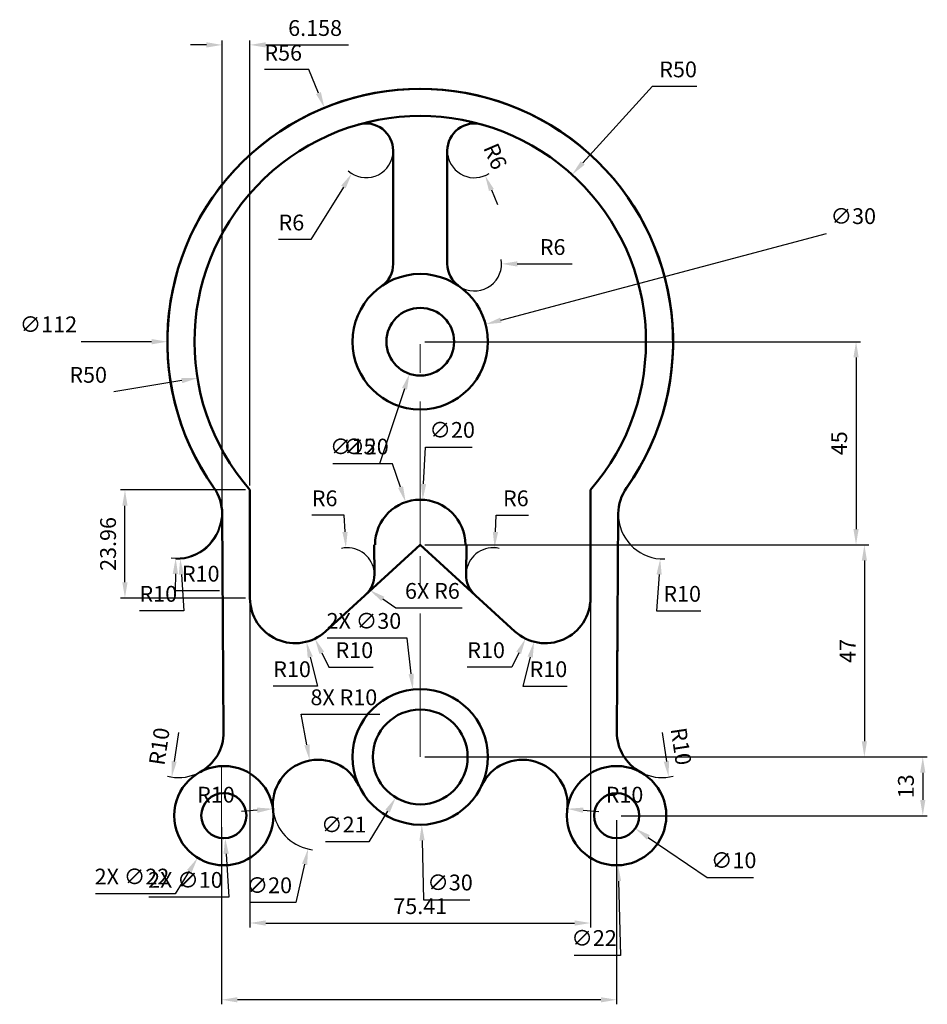
# Model space of a CAD drawing. Units: millimetres. Extents: x 3612 to 3813, y 660 to 878.
import ezdxf

# ---------------------------------------------------------------- set-up
doc = ezdxf.new("R2010")
doc.units = ezdxf.units.MM
doc.linetypes.add('CENTER', pattern=[50.8, 31.75, -6.35, 6.35, -6.35])
for name, color, linetype, lineweight in [('M-CNTR', 4, 'CENTER', 18), ('M-CONS', 8, 'Continuous', 13), ('M-DIMS', 3, 'Continuous', 25), ('M-OUTL', 7, 'Continuous', 50)]:
    doc.layers.add(name, color=color, linetype=linetype, lineweight=lineweight)
doc.styles.get("Standard").update_dxf_attribs({"font": 'arial.ttf'})
doc.dimstyles.new('AM_ISO$0', dxfattribs={"dimtxt": 3.5, "dimasz": 3.5, "dimexe": 1, "dimexo": 1, "dimgap": 1.5, "dimtad": 1, "dimdsep": 46, "dimtxsty": 'Standard', "dimcen": 0, "dimclrd": 256, "dimclre": 256, "dimclrt": 2, "dimadec": 0, "dimazin": 2, "dimtp": 0.1, "dimtm": 0.1, "dimtfac": 0.71, "dimtdec": 3, "dimtmove": 0, "dimatfit": 3, "dimfxl": 1, "dimlwd": -1, "dimlwe": -1, "dimarcsym": 1})
doc.dimstyles.new('AM_ISO$3', dxfattribs={"dimtxt": 3.5, "dimasz": 3.5, "dimexe": 1, "dimexo": 1, "dimgap": 1.5, "dimtad": 1, "dimtoh": 1, "dimdsep": 46, "dimtxsty": 'Standard', "dimcen": 0, "dimclrd": 256, "dimclre": 256, "dimclrt": 2, "dimadec": 0, "dimazin": 2, "dimtp": 0.1, "dimtm": 0.1, "dimtfac": 0.71, "dimtdec": 3, "dimtofl": 0, "dimtmove": 0, "dimatfit": 0, "dimfxl": 1, "dimlwd": -1, "dimlwe": -1, "dimarcsym": 1})
doc.dimstyles.new('AM_ISO$4', dxfattribs={"dimtxt": 3.5, "dimasz": 3.5, "dimexe": 1, "dimexo": 1, "dimgap": 1.5, "dimtad": 1, "dimtoh": 1, "dimdsep": 46, "dimtxsty": 'Standard', "dimcen": 0, "dimclrd": 256, "dimclre": 256, "dimclrt": 2, "dimadec": 0, "dimazin": 2, "dimtp": 0.1, "dimtm": 0.1, "dimtfac": 0.71, "dimtdec": 3, "dimtofl": 0, "dimtmove": 0, "dimatfit": 0, "dimfxl": 1, "dimlwd": -1, "dimlwe": -1, "dimarcsym": 1})

# ---------------------------------------------------------------- blocks, each defined once
blk = doc.blocks.new('*D3')
at = {"layer": 'Defpoints', "color": 0, "transparency": 16777216}
for p in [(3723.75, 703.9), (3733.71, 703.03)]:
    blk.add_point(p, dxfattribs=at)
at = {"layer": 'M-DIMS', "color": 0, "linetype": 'ByBlock', "transparency": 16777216}
blk.add_line((3737.2, 702.72), (3740.69, 702.41), dxfattribs=at)
at = {"layer": 'M-DIMS', "color": 0, "transparency": 16777216}
blk.add_solid([(3737.25, 703.3), (3737.15, 702.14), (3733.71, 703.03)], dxfattribs=at)
at = {"layer": 'M-DIMS', "color": 0, "transparency": 16777216, "insert": (3746.36, 705.7), "char_height": 3.5, "attachment_point": 5}
blk.add_mtext('R10', dxfattribs=at)
blk = doc.blocks.new('*D4')
at = {"layer": 'Defpoints', "color": 0, "transparency": 16777216}
for p in [(3689.12, 848.84), (3685.95, 843.75)]:
    blk.add_point(p, dxfattribs=at)
at = {"layer": 'M-DIMS', "color": 0, "linetype": 'ByBlock', "transparency": 16777216}
for p, q in [((3684.11, 840.77), (3676.9, 829.17)), ((3676.9, 829.17), (3669.76, 829.17))]:
    blk.add_line(p, q, dxfattribs=at)
blk.add_arc((3689.12, 848.84), 6, 228.6118, 350.4507, dxfattribs=at)
at = {"layer": 'M-DIMS', "color": 0, "transparency": 16777216}
blk.add_solid([(3683.61, 841.08), (3684.6, 840.47), (3685.95, 843.75)], dxfattribs=at)
at = {"layer": 'M-DIMS', "color": 0, "transparency": 16777216, "insert": (3672.58, 832.46), "char_height": 3.5, "attachment_point": 5}
blk.add_mtext('R6', dxfattribs=at)
blk = doc.blocks.new('*D5')
at = {"layer": 'Defpoints', "color": 0, "transparency": 16777216}
for p in [(3754.67, 719.95), (3756.15, 710.06)]:
    blk.add_point(p, dxfattribs=at)
at = {"layer": 'M-DIMS', "color": 0, "linetype": 'ByBlock', "transparency": 16777216}
blk.add_line((3754.67, 719.95), (3755.63, 713.52), dxfattribs=at)
blk.add_arc((3754.67, 719.95), 10, 247.141, 284.2413, dxfattribs=at)
at = {"layer": 'M-DIMS', "color": 0, "transparency": 16777216}
blk.add_solid([(3756.2, 713.61), (3755.05, 713.44), (3756.15, 710.06)], dxfattribs=at)
at = {"layer": 'M-DIMS', "color": 0, "transparency": 16777216, "insert": (3758.46, 716.8), "char_height": 3.5, "attachment_point": 5, "rotation": 278.5117}
blk.add_mtext('R10', dxfattribs=at)
blk = doc.blocks.new('*D6')
at = {"layer": 'Defpoints', "color": 0, "transparency": 16777216}
for p in [(3754.98, 768.37), (3754.27, 758.4)]:
    blk.add_point(p, dxfattribs=at)
at = {"layer": 'M-DIMS', "color": 0, "linetype": 'ByBlock', "transparency": 16777216}
for p, q in [((3754.02, 754.91), (3753.45, 746.91)), ((3753.45, 746.91), (3763.3, 746.91))]:
    blk.add_line(p, q, dxfattribs=at)
blk.add_arc((3754.98, 768.37), 10, 185.3551, 271.654, dxfattribs=at)
at = {"layer": 'M-DIMS', "color": 0, "transparency": 16777216}
blk.add_solid([(3753.44, 754.95), (3754.6, 754.87), (3754.27, 758.4)], dxfattribs=at)
at = {"layer": 'M-DIMS', "color": 0, "transparency": 16777216, "insert": (3759.13, 750.2), "char_height": 3.5, "attachment_point": 5}
blk.add_mtext('R10', dxfattribs=at)
blk = doc.blocks.new('*D7')
at = {"layer": 'Defpoints', "color": 0, "transparency": 16777216}
for p in [(3647.12, 768.57), (3646.95, 758.57)]:
    blk.add_point(p, dxfattribs=at)
at = {"layer": 'M-DIMS', "color": 0, "linetype": 'ByBlock', "transparency": 16777216}
for p, q in [((3646.89, 755.07), (3646.82, 751.37)), ((3646.82, 751.37), (3656.67, 751.37))]:
    blk.add_line(p, q, dxfattribs=at)
blk.add_arc((3647.12, 768.57), 10, 263.2873, 354.2704, dxfattribs=at)
at = {"layer": 'M-DIMS', "color": 0, "transparency": 16777216}
blk.add_solid([(3646.3, 755.08), (3647.47, 755.06), (3646.95, 758.57)], dxfattribs=at)
at = {"layer": 'M-DIMS', "color": 0, "transparency": 16777216, "insert": (3652.5, 754.66), "char_height": 3.5, "attachment_point": 5}
blk.add_mtext('R10', dxfattribs=at)
blk = doc.blocks.new('*D8')
at = {"layer": 'Defpoints', "color": 0, "transparency": 16777216}
for p in [(3728.82, 749.72), (3724.45, 740.73)]:
    blk.add_point(p, dxfattribs=at)
at = {"layer": 'M-DIMS', "color": 0, "linetype": 'ByBlock', "transparency": 16777216}
for p, q in [((3722.92, 737.58), (3721.38, 734.43)), ((3721.38, 734.43), (3711.53, 734.43))]:
    blk.add_line(p, q, dxfattribs=at)
at = {"layer": 'M-DIMS', "color": 0, "transparency": 16777216}
blk.add_solid([(3722.39, 737.83), (3723.44, 737.32), (3724.45, 740.73)], dxfattribs=at)
at = {"layer": 'M-DIMS', "color": 0, "transparency": 16777216, "insert": (3715.71, 737.72), "char_height": 3.5, "attachment_point": 5}
blk.add_mtext('R10', dxfattribs=at)
blk = doc.blocks.new('*D9')
at = {"layer": 'Defpoints', "color": 0, "transparency": 16777216}
for p in [(3717.59, 760.86), (3717.27, 754.87)]:
    blk.add_point(p, dxfattribs=at)
at = {"layer": 'M-DIMS', "color": 0, "linetype": 'ByBlock', "transparency": 16777216}
for p, q in [((3717.77, 764.36), (3717.97, 768.08)), ((3717.97, 768.08), (3725.11, 768.08))]:
    blk.add_line(p, q, dxfattribs=at)
blk.add_arc((3717.27, 754.87), 6, 77.3871, 169.7499, dxfattribs=at)
at = {"layer": 'M-DIMS', "color": 0, "transparency": 16777216}
blk.add_solid([(3717.19, 764.39), (3718.36, 764.33), (3717.59, 760.86)], dxfattribs=at)
at = {"layer": 'M-DIMS', "color": 0, "transparency": 16777216, "insert": (3722.29, 771.36), "char_height": 3.5, "attachment_point": 5}
blk.add_mtext('R6', dxfattribs=at)
blk = doc.blocks.new('*D10')
at = {"layer": 'Defpoints', "color": 0, "transparency": 16777216}
for p in [(3728.82, 749.72), (3726.34, 740.03)]:
    blk.add_point(p, dxfattribs=at)
at = {"layer": 'M-DIMS', "color": 0, "linetype": 'ByBlock', "transparency": 16777216}
for p, q in [((3725.48, 736.64), (3723.83, 730.21)), ((3723.83, 730.21), (3733.68, 730.21))]:
    blk.add_line(p, q, dxfattribs=at)
at = {"layer": 'M-DIMS', "color": 0, "transparency": 16777216}
blk.add_solid([(3724.91, 736.78), (3726.04, 736.5), (3726.34, 740.03)], dxfattribs=at)
at = {"layer": 'M-DIMS', "color": 0, "transparency": 16777216, "insert": (3729.51, 733.5), "char_height": 3.5, "attachment_point": 5}
blk.add_mtext('R10', dxfattribs=at)
blk = doc.blocks.new('*D16')
at = {"layer": 'Defpoints', "color": 0, "transparency": 16777216}
for p in [(3668.52, 703.03), (3678.48, 703.9)]:
    blk.add_point(p, dxfattribs=at)
at = {"layer": 'M-DIMS', "color": 0, "linetype": 'ByBlock', "transparency": 16777216}
blk.add_line((3665.03, 702.72), (3661.55, 702.41), dxfattribs=at)
at = {"layer": 'M-DIMS', "color": 0, "transparency": 16777216}
blk.add_solid([(3664.98, 703.3), (3665.08, 702.14), (3668.52, 703.03)], dxfattribs=at)
at = {"layer": 'M-DIMS', "color": 0, "transparency": 16777216, "insert": (3655.87, 705.7), "char_height": 3.5, "attachment_point": 5}
blk.add_mtext('R10', dxfattribs=at)
blk = doc.blocks.new('*D12')
at = {"layer": 'Defpoints', "color": 0, "transparency": 16777216}
for p in [(3647.57, 719.95), (3646.09, 710.06)]:
    blk.add_point(p, dxfattribs=at)
at = {"layer": 'M-DIMS', "color": 0, "linetype": 'ByBlock', "transparency": 16777216}
blk.add_line((3647.57, 719.95), (3646.61, 713.52), dxfattribs=at)
blk.add_arc((3647.57, 719.95), 10, 255.7587, 292.859, dxfattribs=at)
at = {"layer": 'M-DIMS', "color": 0, "transparency": 16777216}
blk.add_solid([(3646.03, 713.61), (3647.18, 713.44), (3646.09, 710.06)], dxfattribs=at)
at = {"layer": 'M-DIMS', "color": 0, "transparency": 16777216, "insert": (3643.77, 716.8), "char_height": 3.5, "attachment_point": 5, "rotation": 81.4883}
blk.add_mtext('R10', dxfattribs=at)
blk = doc.blocks.new('*D13')
at = {"layer": 'Defpoints', "color": 0, "transparency": 16777216}
for p in [(3647.25, 768.37), (3647.96, 758.4)]:
    blk.add_point(p, dxfattribs=at)
at = {"layer": 'M-DIMS', "color": 0, "linetype": 'ByBlock', "transparency": 16777216}
for p, q in [((3648.21, 754.91), (3648.78, 746.91)), ((3648.78, 746.91), (3638.93, 746.91))]:
    blk.add_line(p, q, dxfattribs=at)
blk.add_arc((3647.25, 768.37), 10, 268.346, 354.6449, dxfattribs=at)
at = {"layer": 'M-DIMS', "color": 0, "transparency": 16777216}
blk.add_solid([(3648.79, 754.95), (3647.63, 754.87), (3647.96, 758.4)], dxfattribs=at)
at = {"layer": 'M-DIMS', "color": 0, "transparency": 16777216, "insert": (3643.11, 750.2), "char_height": 3.5, "attachment_point": 5}
blk.add_mtext('R10', dxfattribs=at)
blk = doc.blocks.new('*D11')
at = {"layer": 'Defpoints', "color": 0, "transparency": 16777216}
for p in [(3673.41, 749.72), (3677.79, 740.73)]:
    blk.add_point(p, dxfattribs=at)
at = {"layer": 'M-DIMS', "color": 0, "linetype": 'ByBlock', "transparency": 16777216}
for p, q in [((3679.32, 737.58), (3680.85, 734.43)), ((3680.85, 734.43), (3690.7, 734.43))]:
    blk.add_line(p, q, dxfattribs=at)
at = {"layer": 'M-DIMS', "color": 0, "transparency": 16777216}
blk.add_solid([(3679.84, 737.83), (3678.79, 737.32), (3677.79, 740.73)], dxfattribs=at)
at = {"layer": 'M-DIMS', "color": 0, "transparency": 16777216, "insert": (3686.53, 737.72), "char_height": 3.5, "attachment_point": 5}
blk.add_mtext('R10', dxfattribs=at)
blk = doc.blocks.new('*D14')
at = {"layer": 'Defpoints', "color": 0, "transparency": 16777216}
for p in [(3684.65, 760.86), (3684.97, 754.87)]:
    blk.add_point(p, dxfattribs=at)
at = {"layer": 'M-DIMS', "color": 0, "linetype": 'ByBlock', "transparency": 16777216}
for p, q in [((3684.26, 768.08), (3677.12, 768.08)), ((3684.46, 764.36), (3684.26, 768.08))]:
    blk.add_line(p, q, dxfattribs=at)
blk.add_arc((3684.97, 754.87), 6, 10.2501, 102.6129, dxfattribs=at)
at = {"layer": 'M-DIMS', "color": 0, "transparency": 16777216}
blk.add_solid([(3685.04, 764.39), (3683.88, 764.33), (3684.65, 760.86)], dxfattribs=at)
at = {"layer": 'M-DIMS', "color": 0, "transparency": 16777216, "insert": (3679.94, 771.36), "char_height": 3.5, "attachment_point": 5}
blk.add_mtext('R6', dxfattribs=at)
blk = doc.blocks.new('*D15')
at = {"layer": 'Defpoints', "color": 0, "transparency": 16777216}
for p in [(3673.41, 749.72), (3675.89, 740.03)]:
    blk.add_point(p, dxfattribs=at)
at = {"layer": 'M-DIMS', "color": 0, "linetype": 'ByBlock', "transparency": 16777216}
for p, q in [((3676.76, 736.64), (3678.4, 730.21)), ((3678.4, 730.21), (3668.55, 730.21))]:
    blk.add_line(p, q, dxfattribs=at)
at = {"layer": 'M-DIMS', "color": 0, "transparency": 16777216}
blk.add_solid([(3677.32, 736.78), (3676.19, 736.5), (3675.89, 740.03)], dxfattribs=at)
at = {"layer": 'M-DIMS', "color": 0, "transparency": 16777216, "insert": (3672.73, 733.5), "char_height": 3.5, "attachment_point": 5}
blk.add_mtext('R10', dxfattribs=at)
blk = doc.blocks.new('*D17')
at = {"layer": 'Defpoints', "color": 0, "transparency": 16777216}
for p in [(3701.12, 806.51), (3701.12, 761.51), (3797.64, 761.51)]:
    blk.add_point(p, dxfattribs=at)
at = {"layer": 'M-DIMS', "color": 0, "linetype": 'ByBlock', "transparency": 16777216}
for p, q in [((3702.12, 806.51), (3798.64, 806.51)), ((3797.64, 803.01), (3797.64, 765.01)), ((3702.12, 761.51), (3798.64, 761.51))]:
    blk.add_line(p, q, dxfattribs=at)
at = {"layer": 'M-DIMS', "color": 0, "transparency": 16777216}
for points in [[(3797.06, 803.01), (3798.23, 803.01), (3797.64, 806.51)], [(3797.06, 765.01), (3798.23, 765.01), (3797.64, 761.51)]]:
    blk.add_solid(points, dxfattribs=at)
at = {"layer": 'M-DIMS', "color": 0, "transparency": 16777216, "insert": (3794.36, 784.01), "char_height": 3.5, "attachment_point": 5, "rotation": 90}
blk.add_mtext('45', dxfattribs=at)
blk = doc.blocks.new('*D18')
at = {"layer": 'Defpoints', "color": 0, "transparency": 16777216}
for p in [(3701.12, 761.51), (3701.12, 714.51), (3799.49, 714.51)]:
    blk.add_point(p, dxfattribs=at)
at = {"layer": 'M-DIMS', "color": 0, "linetype": 'ByBlock', "transparency": 16777216}
for p, q in [((3702.12, 761.51), (3800.49, 761.51)), ((3799.49, 758.01), (3799.49, 718.01)), ((3702.12, 714.51), (3800.49, 714.51))]:
    blk.add_line(p, q, dxfattribs=at)
at = {"layer": 'M-DIMS', "color": 0, "transparency": 16777216}
for points in [[(3798.91, 758.01), (3800.07, 758.01), (3799.49, 761.51)], [(3798.91, 718.01), (3800.07, 718.01), (3799.49, 714.51)]]:
    blk.add_solid(points, dxfattribs=at)
at = {"layer": 'M-DIMS', "color": 0, "transparency": 16777216, "insert": (3796.24, 738.01), "char_height": 3.5, "attachment_point": 5, "rotation": 90}
blk.add_mtext('47', dxfattribs=at)
blk = doc.blocks.new('*D19')
at = {"layer": 'Defpoints', "color": 0, "transparency": 16777216}
for p in [(3701.12, 714.51), (3744.62, 701.51), (3812.42, 701.51)]:
    blk.add_point(p, dxfattribs=at)
at = {"layer": 'M-DIMS', "color": 0, "linetype": 'ByBlock', "transparency": 16777216}
for p, q in [((3702.12, 714.51), (3813.42, 714.51)), ((3812.42, 711.01), (3812.42, 705.01)), ((3745.62, 701.51), (3813.42, 701.51))]:
    blk.add_line(p, q, dxfattribs=at)
at = {"layer": 'M-DIMS', "color": 0, "transparency": 16777216}
for points in [[(3811.84, 711.01), (3813.01, 711.01), (3812.42, 714.51)], [(3811.84, 705.01), (3813.01, 705.01), (3812.42, 701.51)]]:
    blk.add_solid(points, dxfattribs=at)
at = {"layer": 'M-DIMS', "color": 0, "transparency": 16777216, "insert": (3809.14, 708.01), "char_height": 3.5, "attachment_point": 5, "rotation": 90}
blk.add_mtext('13', dxfattribs=at)
blk = doc.blocks.new('*D20')
at = {"layer": 'Defpoints', "color": 0, "transparency": 16777216}
for p in [(3744.62, 701.51), (3657.12, 699.99), (3657.12, 660.72)]:
    blk.add_point(p, dxfattribs=at)
at = {"layer": 'M-DIMS', "color": 0, "linetype": 'ByBlock', "transparency": 16777216}
for p, q in [((3744.62, 700.51), (3744.62, 659.72)), ((3657.12, 698.99), (3657.12, 659.72)), ((3741.12, 660.72), (3660.62, 660.72))]:
    blk.add_line(p, q, dxfattribs=at)
at = {"layer": 'M-DIMS', "color": 0, "transparency": 16777216}
for points in [[(3660.62, 661.3), (3660.62, 660.14), (3657.12, 660.72)], [(3741.12, 661.3), (3741.12, 660.14), (3744.62, 660.72)]]:
    blk.add_solid(points, dxfattribs=at)
blk = doc.blocks.new('*D21')
at = {"layer": 'Defpoints', "color": 0, "transparency": 16777216}
for p in [(3713.12, 823.75), (3719.12, 823.75)]:
    blk.add_point(p, dxfattribs=at)
at = {"layer": 'M-DIMS', "color": 0, "linetype": 'ByBlock', "transparency": 16777216}
blk.add_line((3722.62, 823.75), (3734.76, 823.75), dxfattribs=at)
blk.add_arc((3713.12, 823.75), 6, 244.6994, 9.5493, dxfattribs=at)
at = {"layer": 'M-DIMS', "color": 0, "transparency": 16777216}
blk.add_solid([(3722.62, 824.33), (3722.62, 823.16), (3719.12, 823.75)], dxfattribs=at)
at = {"layer": 'M-DIMS', "color": 0, "transparency": 16777216, "insert": (3730.44, 827.03), "char_height": 3.5, "attachment_point": 5}
blk.add_mtext('R6', dxfattribs=at)
blk = doc.blocks.new('*D22')
at = {"layer": 'Defpoints', "color": 0, "transparency": 16777216}
for p in [(3679.9, 858.34), (3701.12, 806.51)]:
    blk.add_point(p, dxfattribs=at)
at = {"layer": 'M-DIMS', "color": 0, "linetype": 'ByBlock', "transparency": 16777216}
for p, q in [((3676.45, 866.78), (3666.59, 866.78)), ((3678.58, 861.58), (3676.45, 866.78))]:
    blk.add_line(p, q, dxfattribs=at)
at = {"layer": 'M-DIMS', "color": 0, "transparency": 16777216}
blk.add_solid([(3679.12, 861.8), (3678.04, 861.36), (3679.9, 858.34)], dxfattribs=at)
at = {"layer": 'M-DIMS', "color": 0, "transparency": 16777216, "insert": (3670.77, 870.07), "char_height": 3.5, "attachment_point": 5}
blk.add_mtext('R56', dxfattribs=at)
blk = doc.blocks.new('*D23')
at = {"layer": 'Defpoints', "color": 0, "transparency": 16777216}
for p in [(3734.75, 843.51), (3701.12, 806.51)]:
    blk.add_point(p, dxfattribs=at)
at = {"layer": 'M-DIMS', "color": 0, "linetype": 'ByBlock', "transparency": 16777216}
for p, q in [((3737.1, 846.1), (3752.55, 863.09)), ((3752.55, 863.09), (3762.4, 863.09))]:
    blk.add_line(p, q, dxfattribs=at)
at = {"layer": 'M-DIMS', "color": 0, "transparency": 16777216}
blk.add_solid([(3736.67, 846.49), (3737.54, 845.71), (3734.75, 843.51)], dxfattribs=at)
at = {"layer": 'M-DIMS', "color": 0, "transparency": 16777216, "insert": (3758.23, 866.38), "char_height": 3.5, "attachment_point": 5}
blk.add_mtext('R50', dxfattribs=at)
blk = doc.blocks.new('*D24')
at = {"layer": 'Defpoints', "color": 0, "transparency": 16777216}
for p in [(3713.12, 848.84), (3715.49, 843.33)]:
    blk.add_point(p, dxfattribs=at)
at = {"layer": 'M-DIMS', "color": 0, "linetype": 'ByBlock', "transparency": 16777216}
blk.add_line((3716.87, 840.12), (3718.26, 836.9), dxfattribs=at)
blk.add_arc((3713.12, 848.84), 6, 189.5493, 302.846, dxfattribs=at)
at = {"layer": 'M-DIMS', "color": 0, "transparency": 16777216}
blk.add_solid([(3717.41, 840.35), (3716.34, 839.89), (3715.49, 843.33)], dxfattribs=at)
at = {"layer": 'M-DIMS', "color": 0, "transparency": 16777216, "insert": (3717.32, 847.39), "char_height": 3.5, "attachment_point": 5, "rotation": 293.2967}
blk.add_mtext('R6', dxfattribs=at)
blk = doc.blocks.new('*D25')
at = {"layer": 'Defpoints', "color": 0, "transparency": 16777216}
for p in [(3715.61, 810.37), (3686.62, 802.65)]:
    blk.add_point(p, dxfattribs=at)
at = {"layer": 'M-DIMS', "color": 0, "linetype": 'ByBlock', "transparency": 16777216}
blk.add_line((3718.99, 811.27), (3791.12, 830.49), dxfattribs=at)
at = {"layer": 'M-DIMS', "color": 0, "transparency": 16777216}
blk.add_solid([(3718.84, 811.84), (3719.14, 810.71), (3715.61, 810.37)], dxfattribs=at)
at = {"layer": 'M-DIMS', "color": 0, "transparency": 16777216, "insert": (3797.03, 833.87), "char_height": 3.5, "attachment_point": 5}
blk.add_mtext('∅30', dxfattribs=at)
blk = doc.blocks.new('*D26')
at = {"layer": 'Defpoints', "color": 0, "transparency": 16777216}
for p in [(3703.49, 813.63), (3698.74, 799.4)]:
    blk.add_point(p, dxfattribs=at)
at = {"layer": 'M-DIMS', "color": 0, "linetype": 'ByBlock', "transparency": 16777216}
for p, q in [((3697.64, 796.08), (3692.09, 779.44)), ((3692.09, 779.44), (3681.74, 779.44))]:
    blk.add_line(p, q, dxfattribs=at)
at = {"layer": 'M-DIMS', "color": 0, "transparency": 16777216}
blk.add_solid([(3697.08, 796.26), (3698.19, 795.89), (3698.74, 799.4)], dxfattribs=at)
at = {"layer": 'M-DIMS', "color": 0, "transparency": 16777216, "insert": (3686.17, 782.82), "char_height": 3.5, "attachment_point": 5}
blk.add_mtext('∅15', dxfattribs=at)
blk = doc.blocks.new('*D27')
at = {"layer": 'Defpoints', "color": 0, "transparency": 16777216}
for p in [(3701.66, 771.5), (3700.58, 751.53)]:
    blk.add_point(p, dxfattribs=at)
at = {"layer": 'M-DIMS', "color": 0, "linetype": 'ByBlock', "transparency": 16777216}
for p, q in [((3701.84, 774.99), (3702.28, 783.13)), ((3702.28, 783.13), (3712.59, 783.13))]:
    blk.add_line(p, q, dxfattribs=at)
at = {"layer": 'M-DIMS', "color": 0, "transparency": 16777216}
blk.add_solid([(3701.26, 775.02), (3702.43, 774.96), (3701.66, 771.5)], dxfattribs=at)
at = {"layer": 'M-DIMS', "color": 0, "transparency": 16777216, "insert": (3708.19, 786.51), "char_height": 3.5, "attachment_point": 5}
blk.add_mtext('∅20', dxfattribs=at)
blk = doc.blocks.new('*D28')
at = {"layer": 'Defpoints', "color": 0, "transparency": 16777216}
for p in [(3700.78, 729.51), (3701.45, 699.52)]:
    blk.add_point(p, dxfattribs=at)
at = {"layer": 'M-DIMS', "color": 0, "linetype": 'ByBlock', "transparency": 16777216}
for p, q in [((3701.53, 696.02), (3701.82, 682.86)), ((3701.82, 682.86), (3712.13, 682.86))]:
    blk.add_line(p, q, dxfattribs=at)
at = {"layer": 'M-DIMS', "color": 0, "transparency": 16777216}
blk.add_solid([(3702.11, 696.03), (3700.94, 696), (3701.45, 699.52)], dxfattribs=at)
at = {"layer": 'M-DIMS', "color": 0, "transparency": 16777216, "insert": (3707.72, 686.25), "char_height": 3.5, "attachment_point": 5}
blk.add_mtext('∅30', dxfattribs=at)
blk = doc.blocks.new('*D29')
at = {"layer": 'Defpoints', "color": 0, "transparency": 16777216}
for p in [(3706.54, 723.5), (3695.69, 705.52)]:
    blk.add_point(p, dxfattribs=at)
at = {"layer": 'M-DIMS', "color": 0, "linetype": 'ByBlock', "transparency": 16777216}
for p, q in [((3693.89, 702.52), (3689.77, 695.69)), ((3689.77, 695.69), (3680.12, 695.69))]:
    blk.add_line(p, q, dxfattribs=at)
at = {"layer": 'M-DIMS', "color": 0, "transparency": 16777216}
blk.add_solid([(3693.39, 702.83), (3694.39, 702.22), (3695.69, 705.52)], dxfattribs=at)
at = {"layer": 'M-DIMS', "color": 0, "transparency": 16777216, "insert": (3684.19, 699.08), "char_height": 3.5, "attachment_point": 5}
blk.add_mtext('∅21', dxfattribs=at)
blk = doc.blocks.new('*D30')
at = {"layer": 'Defpoints', "color": 0, "transparency": 16777216}
for p in [(3744.3, 712.51), (3744.93, 690.52)]:
    blk.add_point(p, dxfattribs=at)
at = {"layer": 'M-DIMS', "color": 0, "linetype": 'ByBlock', "transparency": 16777216}
for p, q in [((3745.03, 687.02), (3745.51, 670.56)), ((3745.51, 670.56), (3735.22, 670.56))]:
    blk.add_line(p, q, dxfattribs=at)
at = {"layer": 'M-DIMS', "color": 0, "transparency": 16777216}
blk.add_solid([(3745.62, 687.04), (3744.45, 687), (3744.93, 690.52)], dxfattribs=at)
at = {"layer": 'M-DIMS', "color": 0, "transparency": 16777216, "insert": (3739.62, 673.95), "char_height": 3.5, "attachment_point": 5}
blk.add_mtext('∅22', dxfattribs=at)
blk = doc.blocks.new('*D31')
at = {"layer": 'Defpoints', "color": 0, "transparency": 16777216}
for p in [(3740.49, 704.34), (3748.74, 698.69)]:
    blk.add_point(p, dxfattribs=at)
at = {"layer": 'M-DIMS', "color": 0, "linetype": 'ByBlock', "transparency": 16777216}
for p, q in [((3751.63, 696.71), (3764.64, 687.78)), ((3764.64, 687.78), (3774.95, 687.78))]:
    blk.add_line(p, q, dxfattribs=at)
at = {"layer": 'M-DIMS', "color": 0, "transparency": 16777216}
blk.add_solid([(3751.96, 697.19), (3751.3, 696.22), (3748.74, 698.69)], dxfattribs=at)
at = {"layer": 'M-DIMS', "color": 0, "transparency": 16777216, "insert": (3770.54, 691.17), "char_height": 3.5, "attachment_point": 5}
blk.add_mtext('∅10', dxfattribs=at)
blk = doc.blocks.new('*D32')
at = {"layer": 'Defpoints', "color": 0, "transparency": 16777216}
for p in [(3680.68, 713.66), (3676.28, 694.15)]:
    blk.add_point(p, dxfattribs=at)
at = {"layer": 'M-DIMS', "color": 0, "linetype": 'ByBlock', "transparency": 16777216}
for p, q in [((3675.51, 690.73), (3673.59, 682.25)), ((3673.59, 682.25), (3663.29, 682.25))]:
    blk.add_line(p, q, dxfattribs=at)
blk.add_arc((3678.48, 703.9), 10, 192.2613, 263.015, dxfattribs=at)
at = {"layer": 'M-DIMS', "color": 0, "transparency": 16777216}
blk.add_solid([(3674.94, 690.86), (3676.08, 690.6), (3676.28, 694.15)], dxfattribs=at)
at = {"layer": 'M-DIMS', "color": 0, "transparency": 16777216, "insert": (3667.69, 685.63), "char_height": 3.5, "attachment_point": 5}
blk.add_mtext('∅20', dxfattribs=at)
blk = doc.blocks.new('MOUNT-BOSS-22-BORE-10')
for radius in [11, 5]:
    blk.add_circle((11, 11), radius)
blk = doc.blocks.new('*D34')
at = {"layer": 'Defpoints', "color": 0, "transparency": 16777216}
for p in [(3663.41, 749.72), (3738.82, 749.72), (3738.82, 677.73)]:
    blk.add_point(p, dxfattribs=at)
at = {"layer": 'M-DIMS', "linetype": 'ByBlock', "transparency": 16777216}
for p, q in [((3663.41, 748.72), (3663.41, 676.73)), ((3738.82, 748.72), (3738.82, 676.73)), ((3666.91, 677.73), (3735.32, 677.73))]:
    blk.add_line(p, q, dxfattribs=at)
at = {"layer": 'M-DIMS', "transparency": 16777216}
for points in [[(3666.91, 678.31), (3666.91, 677.14), (3663.41, 677.73)], [(3735.32, 678.31), (3735.32, 677.14), (3738.82, 677.73)]]:
    blk.add_solid(points, dxfattribs=at)
at = {"layer": 'M-DIMS', "color": 2, "transparency": 16777216, "insert": (3701.12, 681.01), "char_height": 3.5, "attachment_point": 5}
blk.add_mtext('75.41', dxfattribs=at)
blk = doc.blocks.new('*D35')
at = {"layer": 'Defpoints', "color": 0, "transparency": 16777216}
for p in [(3635.72, 773.68), (3663.41, 773.68), (3663.41, 749.72)]:
    blk.add_point(p, dxfattribs=at)
at = {"layer": 'M-DIMS', "linetype": 'ByBlock', "transparency": 16777216}
for p, q in [((3662.41, 773.68), (3634.72, 773.68)), ((3635.72, 753.22), (3635.72, 770.18)), ((3662.41, 749.72), (3634.72, 749.72))]:
    blk.add_line(p, q, dxfattribs=at)
at = {"layer": 'M-DIMS', "transparency": 16777216}
for points in [[(3635.14, 770.18), (3636.3, 770.18), (3635.72, 773.68)], [(3635.14, 753.22), (3636.3, 753.22), (3635.72, 749.72)]]:
    blk.add_solid(points, dxfattribs=at)
at = {"layer": 'M-DIMS', "color": 2, "transparency": 16777216, "insert": (3632.43, 761.7), "char_height": 3.5, "attachment_point": 5, "rotation": 90}
blk.add_mtext('23.96', dxfattribs=at)
blk = doc.blocks.new('*D36')
at = {"layer": 'Defpoints', "color": 0, "transparency": 16777216}
for p in [(3663.41, 872.26), (3663.41, 773.68), (3657.25, 768.44)]:
    blk.add_point(p, dxfattribs=at)
at = {"layer": 'M-DIMS', "linetype": 'ByBlock', "transparency": 16777216}
for p, q in [((3657.25, 769.44), (3657.25, 873.26)), ((3663.41, 774.68), (3663.41, 873.26)), ((3653.75, 872.26), (3650.25, 872.26)), ((3666.91, 872.26), (3685.25, 872.26))]:
    blk.add_line(p, q, dxfattribs=at)
at = {"layer": 'M-DIMS', "transparency": 16777216}
for points in [[(3653.75, 872.85), (3653.75, 871.68), (3657.25, 872.26)], [(3666.91, 872.85), (3666.91, 871.68), (3663.41, 872.26)]]:
    blk.add_solid(points, dxfattribs=at)
at = {"layer": 'M-DIMS', "color": 2, "transparency": 16777216, "insert": (3677.83, 875.55), "char_height": 3.5, "attachment_point": 5}
blk.add_mtext('6.158', dxfattribs=at)
blk = doc.blocks.new('*D37')
at = {"layer": 'Defpoints', "color": 0, "transparency": 16777216}
for p in [(3645.12, 806.51), (3757.12, 806.51)]:
    blk.add_point(p, dxfattribs=at)
at = {"layer": 'M-DIMS', "linetype": 'ByBlock', "transparency": 16777216}
blk.add_line((3641.62, 806.51), (3626.02, 806.51), dxfattribs=at)
at = {"layer": 'M-DIMS', "transparency": 16777216}
blk.add_solid([(3641.62, 807.1), (3641.62, 805.93), (3645.12, 806.51)], dxfattribs=at)
at = {"layer": 'M-DIMS', "color": 2, "transparency": 16777216, "insert": (3618.77, 809.9), "char_height": 3.5, "attachment_point": 5}
blk.add_mtext('∅112', dxfattribs=at)
blk = doc.blocks.new('*D38')
at = {"layer": 'Defpoints', "color": 0, "transparency": 16777216}
for p in [(3701.12, 806.51), (3651.77, 798.45)]:
    blk.add_point(p, dxfattribs=at)
at = {"layer": 'M-DIMS', "linetype": 'ByBlock', "transparency": 16777216}
blk.add_line((3648.32, 797.88), (3633.24, 795.42), dxfattribs=at)
at = {"layer": 'M-DIMS', "transparency": 16777216}
blk.add_solid([(3648.22, 798.46), (3648.41, 797.31), (3651.77, 798.45)], dxfattribs=at)
at = {"layer": 'M-DIMS', "color": 2, "transparency": 16777216, "insert": (3627.57, 798.71), "char_height": 3.5, "attachment_point": 5}
blk.add_mtext('R50', dxfattribs=at)
blk = doc.blocks.new('*D39')
at = {"layer": 'Defpoints', "color": 0, "transparency": 16777216}
for p in [(3699.49, 729.42), (3702.75, 699.6)]:
    blk.add_point(p, dxfattribs=at)
at = {"layer": 'M-DIMS', "linetype": 'ByBlock', "transparency": 16777216}
for p, q in [((3698.24, 740.82), (3680.54, 740.82)), ((3699.11, 732.9), (3698.24, 740.82))]:
    blk.add_line(p, q, dxfattribs=at)
at = {"layer": 'M-DIMS', "transparency": 16777216}
blk.add_solid([(3699.69, 732.97), (3698.53, 732.84), (3699.49, 729.42)], dxfattribs=at)
at = {"layer": 'M-DIMS', "color": 2, "transparency": 16777216, "insert": (3688.64, 744.2), "char_height": 3.5, "attachment_point": 5}
blk.add_mtext('2X ∅30', dxfattribs=at)
blk = doc.blocks.new('*D40')
at = {"layer": 'Defpoints', "color": 0, "transparency": 16777216}
for p in [(3663.42, 710.86), (3651.82, 692.16)]:
    blk.add_point(p, dxfattribs=at)
at = {"layer": 'M-DIMS', "linetype": 'ByBlock', "transparency": 16777216}
for p, q in [((3649.97, 689.19), (3646.86, 684.17)), ((3646.86, 684.17), (3629.18, 684.17))]:
    blk.add_line(p, q, dxfattribs=at)
at = {"layer": 'M-DIMS', "transparency": 16777216}
blk.add_solid([(3649.48, 689.5), (3650.47, 688.88), (3651.82, 692.16)], dxfattribs=at)
at = {"layer": 'M-DIMS', "color": 2, "transparency": 16777216, "insert": (3637.27, 687.56), "char_height": 3.5, "attachment_point": 5}
blk.add_mtext('2X ∅22', dxfattribs=at)
blk = doc.blocks.new('*D41')
at = {"layer": 'Defpoints', "color": 0, "transparency": 16777216}
for p in [(3657.31, 706.5), (3657.92, 696.52)]:
    blk.add_point(p, dxfattribs=at)
at = {"layer": 'M-DIMS', "linetype": 'ByBlock', "transparency": 16777216}
for p, q in [((3658.13, 693.03), (3658.72, 683.43)), ((3658.72, 683.43), (3641.01, 683.43))]:
    blk.add_line(p, q, dxfattribs=at)
at = {"layer": 'M-DIMS', "transparency": 16777216}
blk.add_solid([(3658.72, 693.06), (3657.55, 692.99), (3657.92, 696.52)], dxfattribs=at)
at = {"layer": 'M-DIMS', "color": 2, "transparency": 16777216, "insert": (3649.11, 686.82), "char_height": 3.5, "attachment_point": 5}
blk.add_mtext('2X ∅10', dxfattribs=at)
blk = doc.blocks.new('*D42')
at = {"layer": 'Defpoints', "color": 0, "transparency": 16777216}
for p in [(3684.97, 754.87), (3689.93, 751.5)]:
    blk.add_point(p, dxfattribs=at)
at = {"layer": 'M-DIMS', "linetype": 'ByBlock', "transparency": 16777216}
for p, q in [((3692.82, 749.53), (3695.72, 747.56)), ((3695.72, 747.56), (3710.4, 747.56))]:
    blk.add_line(p, q, dxfattribs=at)
at = {"layer": 'M-DIMS', "transparency": 16777216}
blk.add_solid([(3693.15, 750.01), (3692.5, 749.05), (3689.93, 751.5)], dxfattribs=at)
at = {"layer": 'M-DIMS', "color": 2, "transparency": 16777216, "insert": (3703.81, 750.85), "char_height": 3.5, "attachment_point": 5}
blk.add_mtext('6X R6', dxfattribs=at)
blk = doc.blocks.new('*D43')
at = {"layer": 'Defpoints', "color": 0, "transparency": 16777216}
for p in [(3676.66, 713.73), (3678.48, 703.9)]:
    blk.add_point(p, dxfattribs=at)
at = {"layer": 'M-DIMS', "linetype": 'ByBlock', "transparency": 16777216}
for p, q in [((3676.02, 717.18), (3674.76, 723.99)), ((3674.76, 723.99), (3692.14, 723.99))]:
    blk.add_line(p, q, dxfattribs=at)
at = {"layer": 'M-DIMS', "transparency": 16777216}
blk.add_solid([(3676.6, 717.28), (3675.45, 717.07), (3676.66, 713.73)], dxfattribs=at)
at = {"layer": 'M-DIMS', "color": 2, "transparency": 16777216, "insert": (3684.2, 727.28), "char_height": 3.5, "attachment_point": 5}
blk.add_mtext('8X R10', dxfattribs=at)
blk = doc.blocks.new('*D44')
at = {"layer": 'Defpoints', "color": 0, "transparency": 16777216}
for p in [(3697.89, 770.98), (3704.35, 752.05)]:
    blk.add_point(p, dxfattribs=at)
at = {"layer": 'M-DIMS', "linetype": 'ByBlock', "transparency": 16777216}
for p, q in [((3695, 779.44), (3684.69, 779.44)), ((3696.76, 774.29), (3695, 779.44))]:
    blk.add_line(p, q, dxfattribs=at)
at = {"layer": 'M-DIMS', "transparency": 16777216}
blk.add_solid([(3697.31, 774.48), (3696.21, 774.1), (3697.89, 770.98)], dxfattribs=at)
at = {"layer": 'M-DIMS', "color": 2, "transparency": 16777216, "insert": (3689.1, 782.82), "char_height": 3.5, "attachment_point": 5}
blk.add_mtext('∅20', dxfattribs=at)

msp = doc.modelspace()

# ---------------------------------------------------------------- linework, layer by layer
at = {"layer": 'M-CNTR'}
for p, q in [((3701.1166, 761.5125), (3701.1166, 806.5125)), ((3701.1166, 714.5125), (3701.1166, 761.5125))]:
    msp.add_line(p, q, dxfattribs=at)
at = {"layer": 'M-CONS'}
for p, q in [((3744.7833, 738.0125), (3745.1166, 738.0125)), ((3745.1166, 738.0125), (3744.7833, 738.0125)), ((3657.1166, 712.5011), (3657.1166, 687.4771))]:
    msp.add_line(p, q, dxfattribs=at)
at = {"layer": 'M-OUTL'}
for p, q in [((3695.1166, 823.7461), (3695.1166, 848.8445)), ((3707.1166, 823.7461), (3707.1166, 848.8445)), ((3663.4093, 773.6771), (3663.4093, 749.718)), ((3738.8239, 773.6771), (3738.8239, 749.718)), ((3657.2511, 768.4396), (3657.5676, 720.0175)), ((3744.9822, 768.4396), (3744.6657, 720.0175)), ((3701.1166, 761.5125), (3680.1593, 742.3398)), ((3690.8862, 761.5125), (3690.9666, 754.9435)), ((3701.1166, 761.5125), (3722.074, 742.3398)), ((3711.1166, 761.5125), (3711.347, 761.5125)), ((3711.347, 761.5125), (3711.2667, 754.9435))]:
    msp.add_line(p, q, dxfattribs=at)
for centre, radius in [((3701.1166, 806.5125), 15), ((3701.1166, 806.5125), 7.5), ((3701.1166, 714.5125), 15), ((3701.1166, 714.5125), 15), ((3701.1166, 714.5125), 10.5), ((3701.1166, 714.5125), 10.5)]:
    msp.add_circle(centre, radius, dxfattribs=at)
for centre, radius, start, end in [((3701.1166, 806.5125), 56, 324.700394, 215.096801), ((3701.1166, 806.5125), 56, 324.903199, 215.299606), ((3701.1166, 806.5125), 50, 318.950815, 221.049185), ((3689.1166, 848.8445), 6, 0, 105.82662), ((3713.1166, 848.8445), 6, 74.17338, 180), ((3689.1166, 823.7461), 6, 304.849905, 360), ((3713.1166, 823.7461), 6, 180, 235.150095), ((3647.2513, 768.3742), 10, 0.374497, 35.299606), ((3754.982, 768.3742), 10, 144.700394, 179.625503), ((3701.1166, 761.5125), 10, 0, 180), ((3701.1166, 761.5125), 10, 0, 90), ((3684.967, 754.8701), 6, 312.453604, 0.700831), ((3717.2662, 754.8701), 6, 179.299169, 227.546396), ((3673.4093, 749.718), 10, 180, 312.453604), ((3728.8239, 749.718), 10, 227.546396, 0), ((3647.5678, 719.9521), 10, 298.588541, 0.374497), ((3754.6655, 719.9521), 10, 179.625503, 241.411459), ((3678.4803, 703.9013), 10, 25.115726, 186.531672), ((3723.7529, 703.9013), 10, 353.468328, 154.884274)]:
    msp.add_arc(centre, radius, start, end, dxfattribs=at)

# ---------------------------------------------------------------- block references
for p in [(3646.6166, 690.5125), (3733.6166, 690.5125)]:
    msp.add_blockref('MOUNT-BOSS-22-BORE-10', p, dxfattribs=at)

# ---------------------------------------------------------------- dimensions: what is measured, and where the dimension line sits
at = {"layer": 'M-DIMS'}
for base, p1, p2, override, picture, middle in [((3663.4093, 872.2624), (3657.2511, 768.4396), (3663.4093, 773.6771), {"dimdec": 3, "dimlfac": 1, "dimrnd": 0, "dimzin": 0, "dimdsep": 46, "dimlunit": 2}, '*D36', (3677.8278, 875.5494)), ((3738.8239, 677.7271), (3663.4093, 749.718), (3738.8239, 749.718), {"dimdec": 2, "dimlfac": 1, "dimrnd": 0, "dimzin": 0, "dimdsep": 46, "dimlunit": 2}, '*D34', (3701.1166, 681.0141))]:
    dim = msp.add_linear_dim(base=base, p1=p1, p2=p2, dimstyle='AM_ISO$4', override=override, dxfattribs=at)
    dim.commit()
    dim.dimension.update_dxf_attribs({"geometry": picture, "text_midpoint": middle})
for center, mpoint, override, picture, middle in [((3701.1166, 806.5125), (3679.9046, 858.3396), {"dimclrd": 0, "dimclre": 0, "dimclrt": 0}, '*D22', (3670.7695, 866.7804)), ((3701.1166, 806.5125), (3734.7502, 843.5095), {"dimclrd": 0, "dimclre": 0, "dimclrt": 0}, '*D23', (3758.2261, 863.0897)), ((3713.1166, 848.8445), (3715.4896, 843.3337), {"dimclrd": 0, "dimclre": 0, "dimclrt": 0}, '*D24', (3714.3031, 846.0891)), ((3689.1166, 848.8445), (3685.9514, 843.7473), {"dimpost": '', "dimclrd": 0, "dimclre": 0, "dimclrt": 0}, '*D4', (3672.5801, 829.1724)), ((3713.1166, 823.7461), (3719.1166, 823.7461), {"dimpost": '', "dimclrd": 0, "dimclre": 0, "dimclrt": 0}, '*D21', (3730.4374, 823.7461)), ((3701.1166, 806.5125), (3651.7712, 798.4482), {"dimdec": 0, "dimlfac": 1, "dimrnd": 0, "dimzin": 0, "dimdsep": 46, "dimlunit": 2}, '*D38', (3627.565, 795.4198)), ((3684.967, 754.8701), (3684.6464, 760.8616), {"dimpost": '', "dimclrd": 0, "dimclre": 0, "dimclrt": 0}, '*D14', (3679.9394, 768.0771)), ((3717.2662, 754.8701), (3717.5869, 760.8616), {"dimpost": '', "dimclrd": 0, "dimclre": 0, "dimclrt": 0}, '*D9', (3722.2939, 768.0771)), ((3647.2513, 768.3742), (3647.962, 758.3995), {"dimpost": '', "dimclrd": 0, "dimclre": 0, "dimclrt": 0}, '*D13', (3643.1051, 746.9091)), ((3647.1166, 768.5651), (3646.9451, 758.5666), {"dimpost": '', "dimclrd": 0, "dimclre": 0, "dimclrt": 0}, '*D7', (3652.4973, 751.3729)), ((3754.982, 768.3742), (3754.2713, 758.3995), {"dimpost": '', "dimclrd": 0, "dimclre": 0, "dimclrt": 0}, '*D6', (3759.1282, 746.9091)), ((3673.4093, 749.718), (3675.8894, 740.0304), {"dimpost": '', "dimclrd": 0, "dimclre": 0, "dimclrt": 0}, '*D15', (3672.7277, 730.2105)), ((3673.4093, 749.718), (3677.786, 740.7266), {"dimpost": '', "dimclrd": 0, "dimclre": 0, "dimclrt": 0}, '*D11', (3686.5252, 734.4326)), ((3728.8239, 749.718), (3724.4473, 740.7266), {"dimpost": '', "dimclrd": 0, "dimclre": 0, "dimclrt": 0}, '*D8', (3715.708, 734.4326)), ((3728.8239, 749.718), (3726.3438, 740.0304), {"dimpost": '', "dimclrd": 0, "dimclre": 0, "dimclrt": 0}, '*D10', (3729.5055, 730.2105)), ((3647.5678, 719.9521), (3646.0877, 710.0623), {"dimpost": '', "dimclrd": 0, "dimclre": 0, "dimclrt": 0}, '*D12', (3647.0234, 716.3143)), ((3754.6655, 719.9521), (3756.1456, 710.0623), {"dimpost": '', "dimclrd": 0, "dimclre": 0, "dimclrt": 0}, '*D5', (3755.2099, 716.3143)), ((3678.4803, 703.9013), (3668.5187, 703.0258), {"dimpost": '', "dimclrd": 0, "dimclre": 0, "dimclrt": 0}, '*D16', (3655.8699, 702.4131)), ((3723.7529, 703.9013), (3733.7145, 703.0258), {"dimpost": '', "dimclrd": 0, "dimclre": 0, "dimclrt": 0}, '*D3', (3746.3633, 702.4131))]:
    dim = msp.add_radius_dim(center=center, mpoint=mpoint, dimstyle='AM_ISO$4', override=override, dxfattribs=at)
    dim.commit()
    dim.dimension.update_dxf_attribs({"geometry": picture, "text_midpoint": middle, "dimtype": 164})
for p1, p2, dimstyle, override, picture, middle in [((3686.6221, 802.6513), (3715.6112, 810.3736), 'AM_ISO$3', {"dimpost": '', "dimclrd": 0, "dimclre": 0, "dimclrt": 0}, '*D25', (3797.0273, 830.4891)), ((3703.4884, 813.6276), (3698.7449, 799.3973), 'AM_ISO$3', {"dimclrd": 0, "dimclre": 0, "dimclrt": 0}, '*D26', (3686.1668, 779.4352)), ((3757.1166, 806.513), (3645.1166, 806.5119), 'AM_ISO$4', {"dimdec": 0, "dimlfac": 1, "dimrnd": 0, "dimzin": 0, "dimdsep": 46, "dimlunit": 2}, '*D37', (3618.7692, 806.5117)), ((3700.5778, 751.527), (3701.6554, 771.4979), 'AM_ISO$3', {"dimclrd": 0, "dimclre": 0, "dimclrt": 0}, '*D27', (3708.1877, 783.1258)), ((3704.3458, 752.0482), (3697.8875, 770.9767), 'AM_ISO$4', {"dimdec": 0, "dimlfac": 1, "dimrnd": 0, "dimzin": 0, "dimdsep": 46, "dimlunit": 2}, '*D44', (3689.0957, 779.438)), ((3700.7842, 729.5088), (3701.449, 699.5161), 'AM_ISO$3', {"dimclrd": 0, "dimclre": 0, "dimclrt": 0}, '*D28', (3707.723, 682.8634)), ((3706.5398, 723.5035), (3695.6934, 705.5214), 'AM_ISO$3', {"dimclrd": 0, "dimclre": 0, "dimclrt": 0}, '*D29', (3684.1922, 695.6931)), ((3680.6813, 713.656), (3676.2794, 694.1465), 'AM_ISO$3', {"dimclrd": 0, "dimclre": 0, "dimclrt": 0}, '*D32', (3667.69, 682.2483)), ((3744.2994, 712.5079), (3744.9338, 690.517), 'AM_ISO$3', {"dimclrd": 0, "dimclre": 0, "dimclrt": 0}, '*D30', (3739.6166, 670.5613)), ((3740.4928, 704.3399), (3748.7404, 698.685), 'AM_ISO$3', {"dimclrd": 0, "dimclre": 0, "dimclrt": 0}, '*D31', (3770.5439, 687.7843))]:
    dim = msp.add_diameter_dim_2p(p1=p1, p2=p2, dimstyle=dimstyle, override=override, dxfattribs=at)
    dim.commit()
    dim.dimension.update_dxf_attribs({"geometry": picture, "text_midpoint": middle, "dimtype": 163})
for base, p1, p2, dimstyle, override, picture, middle in [((3797.6431, 761.5125), (3701.1166, 806.5125), (3701.1166, 761.5125), 'AM_ISO$0', {"dimpost": '', "dimclrd": 0, "dimclre": 0, "dimclrt": 0}, '*D17', (3794.3633, 784.0125)), ((3635.7192, 773.6771), (3663.4093, 749.718), (3663.4093, 773.6771), 'AM_ISO$4', {"dimdec": 2, "dimlfac": 1, "dimrnd": 0, "dimzin": 0, "dimdsep": 46, "dimlunit": 2}, '*D35', (3632.431, 761.6976)), ((3799.4908, 714.5125), (3701.1166, 761.5125), (3701.1166, 714.5125), 'AM_ISO$0', {"dimclrd": 0, "dimclre": 0, "dimclrt": 0}, '*D18', (3796.2408, 738.0125)), ((3812.4245, 701.5125), (3701.1166, 714.5125), (3744.6166, 701.5125), 'AM_ISO$0', {"dimclrd": 0, "dimclre": 0, "dimclrt": 0}, '*D19', (3809.1363, 708.0125))]:
    dim = msp.add_linear_dim(base=base, p1=p1, p2=p2, angle=90, dimstyle=dimstyle, override=override, dxfattribs=at)
    dim.commit()
    dim.dimension.update_dxf_attribs({"geometry": picture, "text_midpoint": middle})
for center, mpoint, text, picture, middle in [((3684.967, 754.8701), (3689.9287, 751.4965), '6X <>', '*D42', (3703.8079, 747.5605)), ((3678.4803, 703.9013), (3676.6607, 713.7343), '8X <>', '*D43', (3684.2003, 723.9949))]:
    dim = msp.add_radius_dim(center=center, mpoint=mpoint, text=text, dimstyle='AM_ISO$4', override={"dimdec": 0, "dimlfac": 1, "dimrnd": 0, "dimzin": 0, "dimdsep": 46, "dimlunit": 2}, dxfattribs=at)
    dim.commit()
    dim.dimension.update_dxf_attribs({"geometry": picture, "text_midpoint": middle, "dimtype": 164})
for p1, p2, picture, middle in [((3702.7471, 699.6013), (3699.4862, 729.4236), '*D39', (3688.6382, 740.82)), ((3663.4153, 710.86), (3651.818, 692.1649), '*D40', (3637.2696, 684.1717)), ((3657.313, 706.5032), (3657.9203, 696.5217), '*D41', (3649.115, 683.4304))]:
    dim = msp.add_diameter_dim_2p(p1=p1, p2=p2, text='2X <>', dimstyle='AM_ISO$4', override={"dimdec": 0, "dimlfac": 1, "dimrnd": 0, "dimzin": 0, "dimdsep": 46, "dimlunit": 2}, dxfattribs=at)
    dim.commit()
    dim.dimension.update_dxf_attribs({"geometry": picture, "text_midpoint": middle, "dimtype": 163})
dim = msp.add_linear_dim(base=(3657.1166, 660.7196), p1=(3744.6166, 701.5125), p2=(3657.1166, 699.9891), angle=0, text=' ', dimstyle='AM_ISO$0', override={"dimpost": '', "dimclrd": 0, "dimclre": 0, "dimclrt": 0}, dxfattribs=at)
dim.commit()
dim.dimension.update_dxf_attribs({"geometry": '*D20', "text_midpoint": (3700.8666, 660.7196)})

doc.saveas('drawing.dxf')
